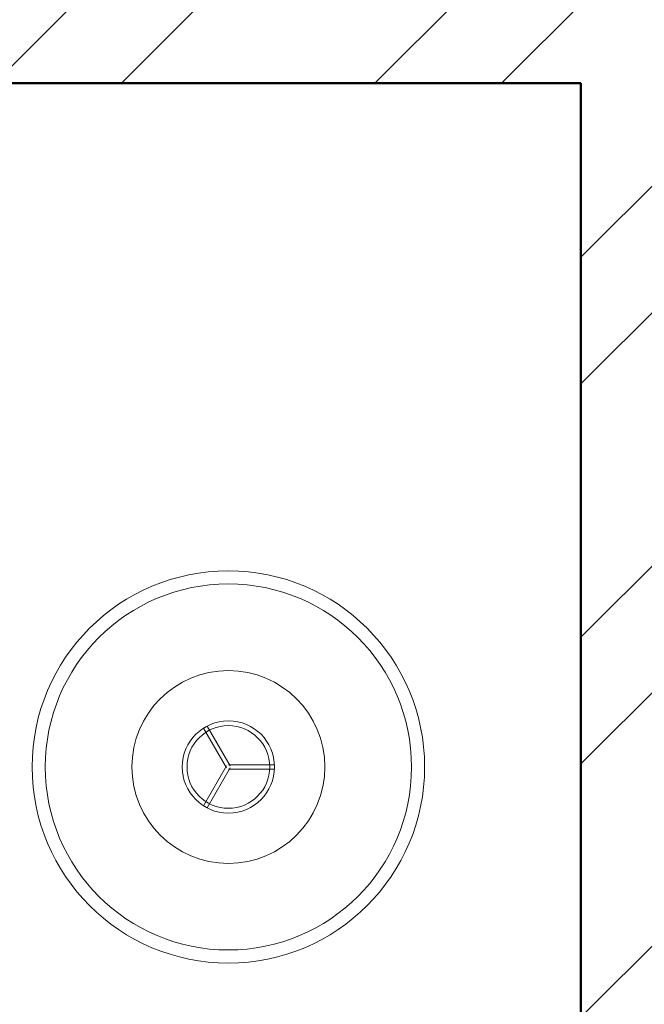
# Model space of a CAD drawing. Units: inches. Extents: x 963 to 2075, y 289 to 2657.
# Tile 79 of 98: x 1489 to 1511, y 2290 to 2325. Entities that reach past the tile are written whole.
import ezdxf

# ---------------------------------------------------------------- set-up
doc = ezdxf.new("R2010")
doc.units = ezdxf.units.IN
for name, color, linetype, lineweight in [('A-FURN', 8, 'Continuous', 18), ('A-WALL', 7, 'Continuous', 50), ('A-WALL-PATT', 8, 'Continuous', 13)]:
    doc.layers.add(name, color=color, linetype=linetype, lineweight=lineweight)

msp = doc.modelspace()

# ---------------------------------------------------------------- hatches: boundary and pattern name
at = {"layer": 'A-WALL-PATT'}
h = msp.add_hatch(dxfattribs=at)
h.set_pattern_fill('ANSI32', color=256)
h.paths.add_polyline_path([(1296.922, 2558.318), (1203.922, 2558.318), (1203.922, 2493.818), (1191.533, 2493.818), (1191.533, 2489.318), (1211.063, 2489.318), (1211.063, 2492.02), (1211.063, 2493.818), (1208.422, 2493.818), (1208.422, 2553.818), (1292.422, 2553.818), (1292.422, 2538.863), (1296.922, 2538.863)])
h.paths.add_polyline_path([(1442.422, 2558.318), (1349.422, 2558.318), (1349.422, 2538.943), (1353.922, 2538.943), (1353.922, 2553.818), (1437.922, 2553.818), (1437.922, 2493.818), (1434.542, 2493.818), (1434.542, 2489.318), (1448.311, 2489.318), (1448.311, 2491.568), (1448.311, 2493.818), (1442.422, 2493.818)])
h.paths.add_polyline_path([(1415.554, 2491.568), (1415.554, 2493.818), (1340.941, 2493.818), (1340.941, 2489.318), (1371.922, 2489.318), (1371.922, 2378.318), (1367.596, 2378.318), (1367.596, 2373.818), (1371.922, 2373.818), (1371.922, 2355.185), (1376.422, 2355.185), (1376.422, 2489.318), (1415.554, 2489.318)])
h.paths.add_polyline_path([(1304.941, 2491.568), (1304.941, 2493.818), (1296.922, 2493.818), (1296.922, 2514.863), (1292.422, 2514.863), (1292.422, 2493.818), (1232.808, 2493.818), (1232.808, 2489.318), (1256.422, 2489.318), (1256.422, 2327.318), (1253.714, 2327.318), (1253.714, 2322.818), (1328.422, 2322.818), (1328.422, 2331.147), (1323.922, 2331.147), (1323.922, 2327.318), (1260.922, 2327.318), (1260.922, 2373.818), (1323.922, 2373.818), (1323.922, 2357.812), (1328.422, 2357.812), (1328.422, 2373.818), (1346.007, 2373.818), (1346.007, 2376.068), (1346.007, 2378.318), (1260.922, 2378.318), (1260.922, 2489.318), (1304.941, 2489.318)])
h.paths.add_polyline_path([(1226.654, 2327.318), (1124.422, 2327.318), (1124.422, 2347.447), (1119.922, 2347.447), (1119.922, 2322.818), (1163.422, 2322.818), (1163.422, 2305.435), (1165.672, 2305.435), (1167.922, 2305.435), (1167.922, 2322.818), (1226.654, 2322.818), (1226.654, 2325.068)])
h.paths.add_polyline_path([(1095.922, 2489.318), (1124.422, 2489.318), (1131.533, 2489.318), (1131.533, 2491.568), (1131.533, 2493.818), (1119.922, 2493.818), (1091.422, 2493.818), (1091.422, 2417.318), (1095.922, 2417.318), (1119.922, 2417.318), (1119.922, 2407.447), (1124.422, 2407.447), (1124.422, 2421.818), (1095.922, 2421.818)])
h.paths.add_polyline_path([(1512.922, 2558.318), (1508.422, 2558.318), (1508.422, 2493.818), (1503.401, 2493.818), (1503.401, 2489.318), (1508.422, 2489.318), (1508.422, 2327.318), (1376.422, 2327.318), (1376.422, 2330.273), (1371.922, 2330.273), (1371.922, 2298.744), (1376.422, 2298.744), (1376.422, 2322.818), (1508.422, 2322.818), (1508.422, 2165.318), (1504.255, 2165.318), (1504.255, 2160.818), (1508.422, 2160.818), (1508.422, 2108.318), (1512.922, 2108.318), (1512.922, 2160.818), (1516.182, 2160.818), (1516.182, 2163.068), (1516.182, 2165.318), (1512.922, 2165.318), (1512.922, 2322.818), (1644.922, 2322.818), (1644.922, 2298.744), (1649.422, 2298.744), (1649.422, 2322.818), (1649.422, 2330.944), (1647.172, 2330.944), (1644.922, 2330.944), (1644.922, 2327.318), (1512.922, 2327.318), (1512.922, 2489.318), (1516.759, 2489.318), (1516.759, 2491.568), (1516.759, 2493.818), (1512.922, 2493.818)])
h.paths.add_polyline_path([(1671.922, 2558.318), (1578.922, 2558.318), (1578.922, 2493.818), (1573.526, 2493.818), (1573.526, 2489.318), (1586.537, 2489.318), (1586.537, 2491.568), (1586.537, 2493.818), (1583.422, 2493.818), (1583.422, 2553.818), (1667.422, 2553.818), (1667.422, 2541.109), (1671.922, 2541.109)])
h.paths.add_polyline_path([(1681.257, 2493.818), (1671.922, 2493.818), (1671.922, 2517.109), (1667.422, 2517.109), (1667.422, 2493.818), (1610.218, 2493.818), (1610.218, 2489.318), (1644.922, 2489.318), (1644.922, 2357.865), (1649.422, 2357.865), (1649.422, 2373.818), (1652.203, 2373.818), (1652.203, 2375.827), (1652.203, 2378.318), (1649.422, 2378.318), (1649.422, 2489.318), (1681.257, 2489.318), (1681.257, 2491.568)])
h.paths.add_polyline_path([(1821.922, 2558.318), (1728.922, 2558.318), (1728.922, 2541), (1733.422, 2541), (1733.422, 2553.818), (1817.422, 2553.818), (1817.422, 2493.818), (1813.507, 2493.818), (1813.507, 2489.318), (1830.078, 2489.318), (1830.078, 2491.568), (1830.078, 2493.818), (1821.922, 2493.818)])
h.paths.add_polyline_path([(1794.244, 2493.818), (1717.257, 2493.818), (1717.257, 2489.318), (1760.422, 2489.318), (1760.422, 2378.318), (1674.401, 2378.318), (1674.401, 2373.818), (1692.922, 2373.818), (1692.922, 2356.954), (1697.422, 2356.954), (1697.422, 2373.818), (1760.422, 2373.818), (1760.422, 2327.318), (1697.422, 2327.318), (1697.422, 2333.341), (1692.922, 2333.341), (1692.922, 2322.818), (1768.037, 2322.818), (1768.037, 2325.068), (1768.037, 2327.318), (1764.922, 2327.318), (1764.922, 2489.318), (1794.244, 2489.318)])
h.paths.add_polyline_path([(1733.422, 2517), (1728.922, 2517), (1728.922, 2493.818), (1733.422, 2493.818)], flags=17)
h.paths.add_polyline_path([(1929.922, 2493.818), (1890.078, 2493.818), (1890.078, 2489.318), (1896.922, 2489.318), (1925.422, 2489.318), (1925.422, 2421.818), (1896.922, 2421.818), (1896.922, 2408.318), (1901.422, 2408.318), (1901.422, 2417.318), (1925.422, 2417.318), (1929.922, 2417.318)])
h.paths.add_polyline_path([(1901.422, 2348.318), (1896.922, 2348.318), (1896.922, 2327.318), (1800.423, 2327.318), (1800.423, 2322.818), (1853.422, 2322.818), (1853.422, 2309.453), (1857.922, 2309.453), (1857.922, 2322.818), (1901.422, 2322.818)])
h.paths.add_polyline_path([(1857.922, 2249.453), (1853.422, 2249.453), (1853.422, 2214.818), (1686.309, 2214.818), (1686.309, 2210.318), (1853.422, 2210.318), (1853.422, 2202.134), (1857.922, 2202.134), (1857.922, 2210.318)])
h.paths.add_polyline_path([(1857.922, 2142.134), (1853.422, 2142.134), (1853.422, 2115.422), (1841.422, 2115.422), (1841.422, 2088.531), (1841.422, 2046.949), (1845.922, 2046.949), (1845.922, 2110.922), (1905.922, 2110.922), (1905.922, 2092.517), (1910.422, 2092.517), (1910.422, 2115.422), (1857.922, 2115.422)])
h.paths.add_polyline_path([(1532.436, 1482.342), (1573.456, 1482.342), (1573.456, 1501), (1532.436, 1501)], flags=9)
h.paths.add_polyline_path([(1438.658, 1486.302), (1479.678, 1486.302), (1479.678, 1504.96), (1438.658, 1504.96)], flags=9)
h.paths.add_polyline_path([(1411.215, 1365.308), (1659.139, 1365.308), (1659.139, 1402.401), (1411.215, 1402.401)], flags=9)
h.paths.add_polyline_path([(1185.671, 2296.298), (1248.16, 2296.298), (1248.16, 2314.955), (1185.671, 2314.955)], flags=9)
h.paths.add_polyline_path([(1177.31, 2187.35), (1216.15, 2187.35), (1216.15, 2206.007), (1177.31, 2206.007)], flags=9)
h.paths.add_polyline_path([(1295.101, 1602.083), (1328.26, 1602.083), (1328.26, 1620.741), (1295.101, 1620.741)], flags=9)
h.paths.add_polyline_path([(1525.126, 2005.99), (1558.39, 2005.99), (1558.39, 2024.648), (1525.126, 2024.648)], flags=9)
h.paths.add_polyline_path([(1459.606, 1977.125), (1472.195, 1977.125), (1472.195, 1987.429), (1459.606, 1987.429)], flags=9)
h.paths.add_polyline_path([(1467.815, 2053.676), (1480.018, 2053.676), (1480.018, 2063.979), (1467.815, 2063.979)], flags=9)
h.paths.add_polyline_path([(1555.184, 2119.02), (1584.563, 2119.02), (1584.563, 2137.678), (1555.184, 2137.678)], flags=25)
h.paths.add_polyline_path([(1405.389, 2115.291), (1444.478, 2115.291), (1444.478, 2133.948), (1405.389, 2133.948)], flags=25)
h.paths.add_polyline_path([(1698.482, 2004.259), (1727.695, 2004.259), (1727.695, 2022.916), (1698.482, 2022.916)], flags=9)
h.paths.add_polyline_path([(1612.158, 1972.855), (1629.016, 1972.855), (1629.016, 1983.159), (1612.158, 1983.159)], flags=9)
h.paths.add_polyline_path([(1608.289, 2060.036), (1625.147, 2060.036), (1625.147, 2070.34), (1608.289, 2070.34)], flags=9)
h.paths.add_polyline_path([(1527.954, 1684.402), (1566.795, 1684.402), (1566.795, 1703.06), (1527.954, 1703.06)], flags=9)
h.paths.add_polyline_path([(1422.792, 1683.59), (1461.633, 1683.59), (1461.633, 1702.247), (1422.792, 1702.247)], flags=9)
h.paths.add_polyline_path([(1531.262, 1732.459), (1574.015, 1732.459), (1574.015, 1751.116), (1531.262, 1751.116)], flags=9)
h.paths.add_polyline_path([(1402.872, 1732.845), (1439.799, 1732.845), (1439.799, 1751.502), (1402.872, 1751.502)], flags=9)
h.paths.add_polyline_path([(1243.122, 1923.132), (1281.962, 1923.132), (1281.962, 1941.79), (1243.122, 1941.79)], flags=9)
h.paths.add_polyline_path([(1181.752, 1792.268), (1244.241, 1792.268), (1244.241, 1810.926), (1181.752, 1810.926)], flags=9)
h.paths.add_polyline_path([(1265.822, 1670.3), (1316.071, 1670.3), (1316.071, 1688.957), (1265.822, 1688.957)], flags=9)
h.paths.add_polyline_path([(1140.263, 1676.054), (1179.104, 1676.054), (1179.104, 1694.711), (1140.263, 1694.711)], flags=9)
h.paths.add_polyline_path([(1107.49, 1490.889), (1143.374, 1490.889), (1143.374, 1509.546), (1107.49, 1509.546)], flags=9)
h.paths.add_polyline_path([(1217.584, 1483.899), (1246.741, 1483.899), (1246.741, 1502.556), (1217.584, 1502.556)], flags=9)
h.paths.add_polyline_path([(1389.21, 1486.919), (1418.367, 1486.919), (1418.367, 1505.576), (1389.21, 1505.576)], flags=9)
h.paths.add_polyline_path([(1672.208, 1602.083), (1705.366, 1602.083), (1705.366, 1620.741), (1672.208, 1620.741)], flags=9)
h.paths.add_polyline_path([(1752.082, 1522.638), (1781.24, 1522.638), (1781.24, 1541.295), (1752.082, 1541.295)], flags=9)
h.paths.add_polyline_path([(1848.275, 1491.26), (1884.158, 1491.26), (1884.158, 1509.918), (1848.275, 1509.918)], flags=9)
h.paths.add_polyline_path([(1822.47, 1685.62), (1861.31, 1685.62), (1861.31, 1704.278), (1822.47, 1704.278)], flags=9)
h.paths.add_polyline_path([(1713.195, 1672.232), (1763.444, 1672.232), (1763.444, 1690.889), (1713.195, 1690.889)], flags=9)
h.paths.add_polyline_path([(1736.619, 1790.578), (1799.109, 1790.578), (1799.109, 1809.235), (1736.619, 1809.235)], flags=9)
h.paths.add_polyline_path([(1691.491, 1916.355), (1730.332, 1916.355), (1730.332, 1935.013), (1691.491, 1935.013)], flags=9)
h.paths.add_polyline_path([(1764.872, 1973.922), (1794.306, 1973.922), (1794.306, 1992.58), (1764.872, 1992.58)], flags=9)
h.paths.add_polyline_path([(1767.854, 2034.017), (1797.288, 2034.017), (1797.288, 2052.674), (1767.854, 2052.674)], flags=9)
h.paths.add_polyline_path([(1851.593, 2060.331), (1880.751, 2060.331), (1880.751, 2078.989), (1851.593, 2078.989)], flags=25)
h.paths.add_polyline_path([(1688.491, 2086.874), (1727.332, 2086.874), (1727.332, 2105.531), (1688.491, 2105.531)], flags=9)
h.paths.add_polyline_path([(1537.743, 2293.581), (1580.495, 2293.581), (1580.495, 2312.239), (1537.743, 2312.239)], flags=25)
h.paths.add_polyline_path([(1425.587, 2296.109), (1468.34, 2296.109), (1468.34, 2314.766), (1425.587, 2314.766)], flags=25)
h.paths.add_polyline_path([(1278.518, 2004.184), (1307.72, 2004.184), (1307.72, 2022.841), (1278.518, 2022.841)], flags=9)
h.paths.add_polyline_path([(1193.282, 1973.635), (1222.715, 1973.635), (1222.715, 1992.292), (1193.282, 1992.292)], flags=9)
h.paths.add_polyline_path([(1192.411, 2040.577), (1221.845, 2040.577), (1221.845, 2059.234), (1192.411, 2059.234)], flags=9)
h.paths.add_polyline_path([(1130.603, 1951.393), (1159.76, 1951.393), (1159.76, 1970.05), (1130.603, 1970.05)], flags=9)
h.paths.add_polyline_path([(1132.827, 2052.494), (1161.984, 2052.494), (1161.984, 2071.151), (1132.827, 2071.151)], flags=9)
h.paths.add_polyline_path([(1265.128, 2334.619), (1315.377, 2334.619), (1315.377, 2353.277), (1265.128, 2353.277)], flags=25)
h.paths.add_polyline_path([(1136.741, 2330.785), (1175.582, 2330.785), (1175.582, 2349.443), (1136.741, 2349.443)], flags=9)
h.paths.add_polyline_path([(1287.422, 2417.204), (1320.58, 2417.204), (1320.58, 2435.861), (1287.422, 2435.861)], flags=25)
h.paths.add_polyline_path([(1430.988, 2329.159), (1469.828, 2329.159), (1469.828, 2347.816), (1430.988, 2347.816)], flags=25)
h.paths.add_polyline_path([(1525.424, 2329.213), (1564.264, 2329.213), (1564.264, 2347.87), (1525.424, 2347.87)], flags=25)
h.paths.add_polyline_path([(1684.525, 2382.799), (1717.683, 2382.799), (1717.683, 2401.457), (1684.525, 2401.457)], flags=25)
h.paths.add_polyline_path([(1704.805, 2340.293), (1755.054, 2340.293), (1755.054, 2358.95), (1704.805, 2358.95)], flags=25)
h.paths.add_polyline_path([(1694.113, 2287.757), (1756.602, 2287.757), (1756.602, 2306.414), (1694.113, 2306.414)], flags=9)
h.paths.add_polyline_path([(1815.778, 2329.861), (1854.618, 2329.861), (1854.618, 2348.518), (1815.778, 2348.518)], flags=9)
h.paths.add_polyline_path([(1842.873, 2514.256), (1878.756, 2514.256), (1878.756, 2532.914), (1842.873, 2532.914)], flags=9)
h.paths.add_polyline_path([(1769.513, 2531.447), (1798.671, 2531.447), (1798.671, 2550.104), (1769.513, 2550.104)], flags=25)
h.paths.add_polyline_path([(1594.772, 2518.468), (1623.93, 2518.468), (1623.93, 2537.125), (1594.772, 2537.125)], flags=25)
h.paths.add_polyline_path([(1520.723, 2516.185), (1556.606, 2516.185), (1556.606, 2534.842), (1520.723, 2534.842)], flags=25)
h.paths.add_polyline_path([(1464.456, 2516.694), (1500.34, 2516.694), (1500.34, 2535.351), (1464.456, 2535.351)], flags=25)
h.paths.add_polyline_path([(1365.696, 2528.97), (1394.854, 2528.97), (1394.854, 2547.627), (1365.696, 2547.627)], flags=25)
h.paths.add_polyline_path([(1222.838, 2516.231), (1251.995, 2516.231), (1251.995, 2534.889), (1222.838, 2534.889)], flags=25)
h.paths.add_polyline_path([(1104.545, 2509.6), (1140.429, 2509.6), (1140.429, 2528.257), (1104.545, 2528.257)], flags=9)

# ---------------------------------------------------------------- linework, layer by layer
at = {"layer": 'A-FURN', "ltscale": 0.03}
for p, q in [((1495.872, 2298.54), (1495.055, 2299.955)), ((1495.998, 2298.613), (1495.181, 2300.028)), ((1495.872, 2298.613), (1495.055, 2297.197)), ((1495.935, 2298.649), (1497.569, 2298.649)), ((1495.998, 2298.54), (1495.181, 2297.124)), ((1495.935, 2298.503), (1497.569, 2298.503))]:
    msp.add_line(p, q, dxfattribs=at)
for radius in [6.953, 3.418, 1.636, 1.466]:
    msp.add_circle((1495.935, 2298.576), radius, dxfattribs=at)
at = {"layer": 'A-FURN'}
msp.add_circle((1495.935, 2298.576), 6.489, dxfattribs=at)
at = {"layer": 'A-WALL'}
for p, q in [((1376.422, 2322.818), (1508.422, 2322.818)), ((1508.422, 2322.818), (1508.422, 2165.318))]:
    msp.add_line(p, q, dxfattribs=at)

doc.saveas('drawing.dxf')
